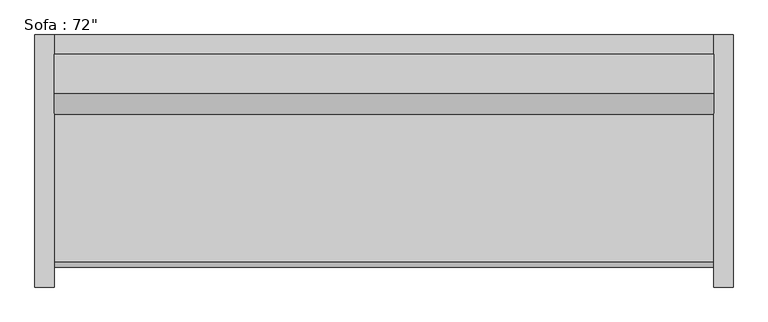
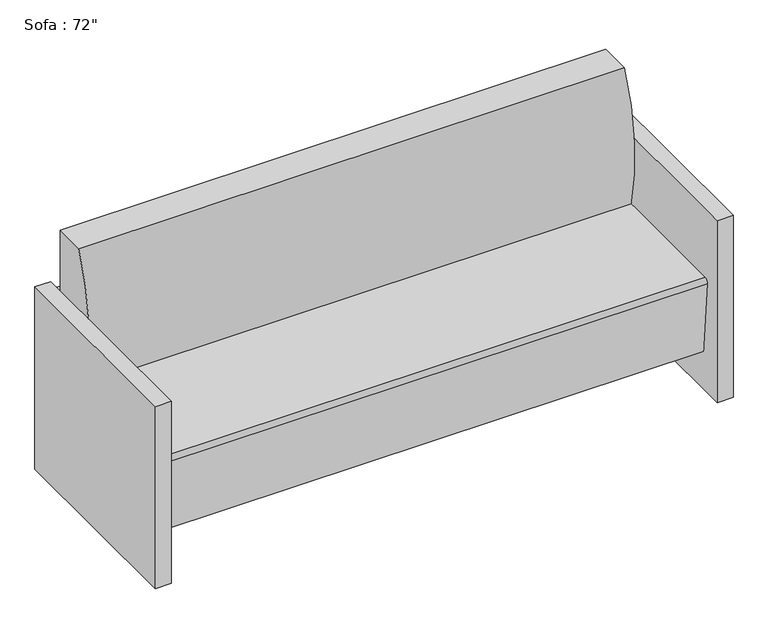
"""IFC4 building model written with IfcOpenShell, lengths in millimetres: furniture geometry."""

from ifc_helpers import new_model, si_unit, point, frame, frame_2d, origin, origin_with_axes, place, context, project, spatial, polyline, circle_curve, trimmed, segment, composite_curve, outline, extrude, source, transform, mapped, element, save


def furniture_57f9710a(model_context):
    return source(origin(), model_context, "Body", "SweptSolid", [
        extrude(outline(polyline([(-844.0295082, 476.3540984), (-793.2295082, 476.3540984), (-793.2295082, -184.0459016), (-844.0295082, -184.0459016), (-844.0295082, 476.3540984)])), origin_with_axes(), (0.0, 0.0, 1.0), 609.6),
        extrude(outline(polyline([(984.7704918, 476.3540984), (984.7704918, -184.0459016), (933.9704918, -184.0459016), (933.9704918, 476.3540984), (984.7704918, 476.3540984)])), origin_with_axes(), (0.0, 0.0, 1.0), 609.6),
        extrude(outline(composite_curve([segment(trimmed(circle_curve(frame_2d((926.517198, 542.5300036)), 660.4), [point((286.1764935, 381.0))], [point((323.9540984, 812.8))], False, "CARTESIAN"), True, "CONTINUOUS"), segment(polyline([(323.9540984, 812.8), (425.5540984, 812.8), (425.5540984, 127.9665467), (-111.108343, 127.9665467), (-132.0379563, 367.1931221)]), True, "CONTINUOUS"), segment(trimmed(circle_curve(frame_2d((-119.3862837, 368.3)), 12.7), [point((-132.0379563, 367.1931221))], [point((-119.3862837, 381.0))], False, "CARTESIAN"), True, "CONTINUOUS"), segment(polyline([(-119.3862837, 381.0), (286.1764935, 381.0)]), True, "CONTINUOUS")], self_intersect=False)), frame((-793.2295082, 0.0, 0.0), z_axis=(1.0, 0.0, 0.0), x_axis=(0.0, 1.0, 0.0)), (0.0, 0.0, 1.0), 1727.2),
        extrude(outline(polyline([(-793.2295082, 425.5540984), (-793.2295082, 476.3540984), (933.9704918, 476.3540984), (933.9704918, 425.5540984), (-793.2295082, 425.5540984)])), frame((0.0, 0.0, 457.2), z_axis=(0.0, 0.0, 1.0), x_axis=(1.0, 0.0, 0.0)), (0.0, 0.0, 1.0), 127.0),
        extrude(outline(polyline([(-793.2295082, 425.5540984), (-793.2295082, 476.3540984), (933.9704918, 476.3540984), (933.9704918, 425.5540984), (-793.2295082, 425.5540984)])), frame((0.0, 0.0, 266.7), z_axis=(0.0, 0.0, 1.0), x_axis=(1.0, 0.0, 0.0)), (0.0, 0.0, 1.0), 127.0),
        extrude(outline(polyline([(-793.2295082, 425.5540984), (-793.2295082, 476.3540984), (933.9704918, 476.3540984), (933.9704918, 425.5540984), (-793.2295082, 425.5540984)])), frame((0.0, 0.0, 76.2), z_axis=(0.0, 0.0, 1.0), x_axis=(1.0, 0.0, 0.0)), (0.0, 0.0, 1.0), 127.0),
    ])


if __name__ == "__main__":
    model = new_model("IFC4")
    model_context = context("Model", 3, world=origin())
    ifc_project = project(units=[si_unit("LENGTHUNIT", "METRE", prefix="MILLI")], contexts=[model_context])
    site = spatial("IfcSite", under=ifc_project)
    building = spatial("IfcBuilding", under=site)
    placement = place(None, origin())
    furniture_shape = furniture_57f9710a(model_context)
    element("IfcFurniture", 1, ObjectType="Sofa : 72\"", at=placement, inside=building, context=model_context, shape_type="MappedRepresentation", body=[
        mapped(furniture_shape, transform((0.0, 0.0, 0.0), x_axis=(1.0, 0.0, 0.0), y_axis=(0.0, 1.0, 0.0), z_axis=(0.0, 0.0, 1.0))),
    ])
    save(model, "model.ifc")

# Revit data of these elements
# Type "Sofa : 72\""
#   Assembly Code = "E2020200"
#   Width = 6' - 0"
#   Seat Material = Linen, Beige
#   Frame Material = Cherry
#   Default Elevation = 0
# Element 1 (IfcFurniture, "Sofa : 72\"")
#   Materials on its faces: "Cherry", "Linen, Beige"
# Materials
#   "Linen, Beige": class "Textile", colour RGB 249 239 230, transparency 0, Description = "Linen, beige", Cost = 0
#   "Cherry": class "Wood", colour RGB 226 177 128, transparency 0, Description = "Prunus Serotina", Cost = 0
